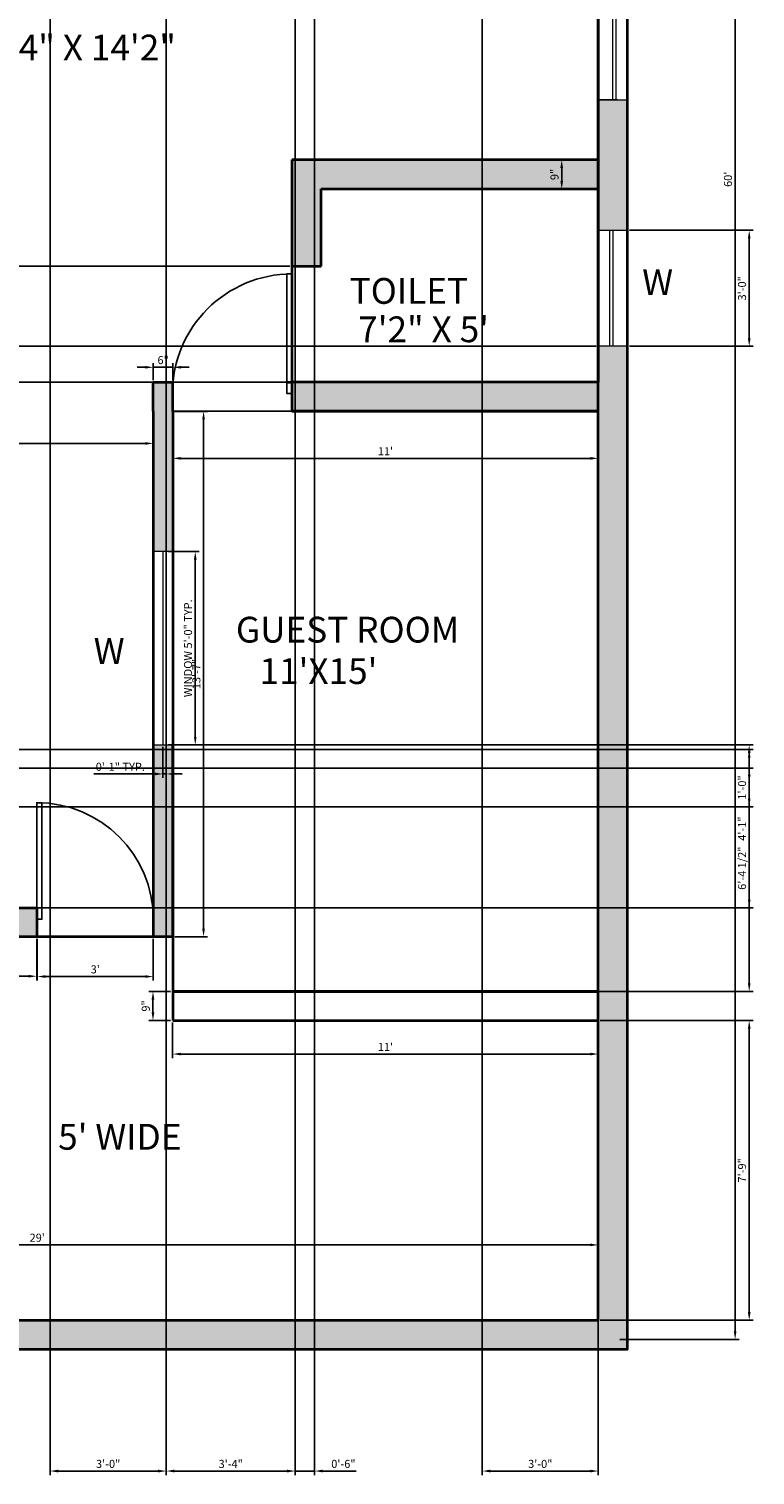
# Model space of a CAD drawing. Units: inches. Extents: x 844 to 1293, y 1224 to 2014.
# Tile 2 of 4: x 1068 to 1293, y 1224 to 1673. Entities that reach past the tile are written whole.
import ezdxf

# ---------------------------------------------------------------- set-up
doc = ezdxf.new("R2010")
doc.units = ezdxf.units.IN
for name, color, linetype, lineweight in [('A-ANNO-DIMS', 2, 'Continuous', 18), ('A-ANNO-TEXT', 3, 'Continuous', 18), ('A-AREA-IDEN', 7, 'Continuous', 25), ('A-DOOR', 3, 'Continuous', 25), ('A-GLAZ', 4, 'Continuous', 18), ('A-WALL', 7, 'Continuous', 35), ('A-WALL-PATT', 252, 'Continuous', 13)]:
    doc.layers.add(name, color=color, linetype=linetype, lineweight=lineweight)
doc.styles.get("Standard").update_dxf_attribs({"font": 'arial.ttf'})
doc.dimstyles.new('Copy of ISO-25', dxfattribs={"dimtxt": 2.5, "dimasz": 2.5, "dimexe": 1.25, "dimexo": 0.625, "dimtad": 1, "dimlunit": 4, "dimtxsty": 'Standard', "dimcen": 2.5, "dimadec": 0, "dimazin": 0, "dimtfac": 1, "dimtmove": 0, "dimatfit": 3, "dimfxl": 1, "dimarcsym": 0})

# ---------------------------------------------------------------- blocks, each defined once
blk = doc.blocks.new('*U3')
for p, q in [((0, 0), (0, -6)), ((40, 0), (40, -6))]:
    blk.add_line(p, q)
blk.add_lwpolyline([(0, 0), (0, 40), (1.75, 40), (1.75, 0)], close=True)
blk.add_arc((0, 0), 40, 0, 90)
blk = doc.blocks.new('*U2')
for p, q in [((0, 0), (0, -6)), ((-40, 0), (-40, -6))]:
    blk.add_line(p, q)
blk.add_lwpolyline([(0, 0), (0, 40), (-1.75, 40), (-1.75, 0)], close=True)
blk.add_arc((0, 0), 40, 90, 180)
blk = doc.blocks.new('*D17')
at = {"layer": 'A-ANNO-DIMS', "color": 0, "lineweight": -2, "transparency": 16777216}
for p, q in [((998.46, 1553.35), (998.46, 1542.83)), ((1106.46, 1553.35), (1106.46, 1542.83)), ((1000.96, 1544.08), (1103.96, 1544.08))]:
    blk.add_line(p, q, dxfattribs=at)
at = {"layer": 'A-ANNO-DIMS', "color": 0, "transparency": 16777216}
for points in [[(1000.96, 1544.49), (1000.96, 1543.66), (998.46, 1544.08)], [(1103.96, 1544.49), (1103.96, 1543.66), (1106.46, 1544.08)]]:
    blk.add_solid(points, dxfattribs=at)
at = {"layer": 'Defpoints', "color": 0, "transparency": 16777216}
for p in [(998.46, 1553.98), (1106.46, 1553.98), (1106.46, 1544.08)]:
    blk.add_point(p, dxfattribs=at)
at = {"layer": 'A-ANNO-DIMS', "color": 0, "transparency": 16777216, "insert": (1052.46, 1545.98), "char_height": 2.5, "attachment_point": 5}
blk.add_mtext("9'", dxfattribs=at)
blk = doc.blocks.new('*D20')
at = {"layer": 'A-ANNO-DIMS', "color": 0, "lineweight": -2, "transparency": 16777216}
for p, q in [((1251.09, 1986.04), (1288.15, 1986.04)), ((1286.9, 1983.54), (1286.9, 1268.54)), ((1251.09, 1266.04), (1288.15, 1266.04))]:
    blk.add_line(p, q, dxfattribs=at)
at = {"layer": 'A-ANNO-DIMS', "color": 0, "transparency": 16777216}
for points in [[(1286.48, 1983.54), (1287.31, 1983.54), (1286.9, 1986.04)], [(1286.48, 1268.54), (1287.31, 1268.54), (1286.9, 1266.04)]]:
    blk.add_solid(points, dxfattribs=at)
at = {"layer": 'Defpoints', "color": 0, "transparency": 16777216}
for p in [(1250.46, 1986.04), (1250.46, 1266.04), (1286.9, 1266.04)]:
    blk.add_point(p, dxfattribs=at)
at = {"layer": 'A-ANNO-DIMS', "color": 0, "transparency": 16777216, "insert": (1285, 1626.04), "char_height": 2.5, "attachment_point": 5, "rotation": 90}
blk.add_mtext("60'", dxfattribs=at)
blk = doc.blocks.new('*D21')
at = {"layer": 'A-ANNO-DIMS', "color": 0, "lineweight": -2, "transparency": 16777216}
for p, q in [((989.46, 1390.05), (989.46, 1377.52)), ((1070.31, 1390.42), (1070.31, 1377.52)), ((991.96, 1378.77), (1067.81, 1378.77))]:
    blk.add_line(p, q, dxfattribs=at)
at = {"layer": 'A-ANNO-DIMS', "color": 0, "transparency": 16777216}
for points in [[(991.96, 1379.19), (991.96, 1378.36), (989.46, 1378.77)], [(1067.81, 1379.19), (1067.81, 1378.36), (1070.31, 1378.77)]]:
    blk.add_solid(points, dxfattribs=at)
at = {"layer": 'Defpoints', "color": 0, "transparency": 16777216}
for p in [(1070.31, 1391.04), (989.46, 1390.68), (1070.31, 1378.77)]:
    blk.add_point(p, dxfattribs=at)
at = {"layer": 'A-ANNO-DIMS', "color": 0, "transparency": 16777216, "insert": (1029.89, 1382.36), "char_height": 2.5, "attachment_point": 5}
blk.add_mtext('6\'-8{\\H1x;\\S3/4;}"', dxfattribs=at)
blk = doc.blocks.new('*D22')
at = {"layer": 'A-ANNO-DIMS', "color": 0, "lineweight": -2, "transparency": 16777216}
for p, q in [((1070.46, 1390.42), (1070.46, 1377.42)), ((1106.46, 1390.42), (1106.46, 1377.42)), ((1072.96, 1378.67), (1103.96, 1378.67))]:
    blk.add_line(p, q, dxfattribs=at)
at = {"layer": 'A-ANNO-DIMS', "color": 0, "transparency": 16777216}
for points in [[(1072.96, 1379.09), (1072.96, 1378.26), (1070.46, 1378.67)], [(1103.96, 1379.09), (1103.96, 1378.26), (1106.46, 1378.67)]]:
    blk.add_solid(points, dxfattribs=at)
at = {"layer": 'Defpoints', "color": 0, "transparency": 16777216}
for p in [(1070.46, 1391.04), (1106.46, 1391.04), (1106.46, 1378.67)]:
    blk.add_point(p, dxfattribs=at)
at = {"layer": 'A-ANNO-DIMS', "color": 0, "transparency": 16777216, "insert": (1088.46, 1380.57), "char_height": 2.5, "attachment_point": 5}
blk.add_mtext("3'", dxfattribs=at)
blk = doc.blocks.new('*D23')
at = {"layer": 'A-ANNO-DIMS', "color": 0, "lineweight": -2, "transparency": 16777216}
for p, q in [((1111.84, 1374.04), (1105.1, 1374.04)), ((1106.35, 1367.54), (1106.35, 1371.54)), ((1111.84, 1365.04), (1105.1, 1365.04))]:
    blk.add_line(p, q, dxfattribs=at)
at = {"layer": 'A-ANNO-DIMS', "color": 0, "transparency": 16777216}
for points in [[(1105.93, 1371.54), (1106.77, 1371.54), (1106.35, 1374.04)], [(1105.93, 1367.54), (1106.77, 1367.54), (1106.35, 1365.04)]]:
    blk.add_solid(points, dxfattribs=at)
at = {"layer": 'Defpoints', "color": 0, "transparency": 16777216}
for p in [(1106.35, 1374.04), (1112.46, 1374.04), (1112.46, 1365.04)]:
    blk.add_point(p, dxfattribs=at)
at = {"layer": 'A-ANNO-DIMS', "color": 0, "transparency": 16777216, "insert": (1104.45, 1369.54), "char_height": 2.5, "attachment_point": 5, "rotation": 90}
blk.add_mtext('9"', dxfattribs=at)
blk = doc.blocks.new('*D24')
at = {"layer": 'A-ANNO-DIMS', "color": 0, "lineweight": -2, "transparency": 16777216}
for p, q in [((1112.46, 1364.42), (1112.46, 1353.37)), ((1244.46, 1364.42), (1244.46, 1353.37)), ((1114.96, 1354.62), (1241.96, 1354.62))]:
    blk.add_line(p, q, dxfattribs=at)
at = {"layer": 'A-ANNO-DIMS', "color": 0, "transparency": 16777216}
for points in [[(1114.96, 1355.04), (1114.96, 1354.2), (1112.46, 1354.62)], [(1241.96, 1355.04), (1241.96, 1354.2), (1244.46, 1354.62)]]:
    blk.add_solid(points, dxfattribs=at)
at = {"layer": 'Defpoints', "color": 0, "transparency": 16777216}
for p in [(1112.46, 1365.04), (1244.46, 1365.04), (1244.46, 1354.62)]:
    blk.add_point(p, dxfattribs=at)
at = {"layer": 'A-ANNO-DIMS', "color": 0, "transparency": 16777216, "insert": (1178.46, 1356.5), "char_height": 2.5, "attachment_point": 5}
blk.add_mtext("11'", dxfattribs=at)
blk = doc.blocks.new('*D31')
at = {"layer": 'A-ANNO-DIMS', "color": 0, "lineweight": -2, "transparency": 16777216}
for p, q in [((896.46, 1272.67), (896.46, 1296.66)), ((1241.96, 1295.41), (898.96, 1295.41)), ((1244.46, 1272.67), (1244.46, 1296.66))]:
    blk.add_line(p, q, dxfattribs=at)
at = {"layer": 'A-ANNO-DIMS', "color": 0, "transparency": 16777216}
for points in [[(898.96, 1295.83), (898.96, 1295), (896.46, 1295.41)], [(1241.96, 1295.83), (1241.96, 1295), (1244.46, 1295.41)]]:
    blk.add_solid(points, dxfattribs=at)
at = {"layer": 'Defpoints', "color": 0, "transparency": 16777216}
for p in [(896.46, 1295.41), (896.46, 1272.04), (1244.46, 1272.04)]:
    blk.add_point(p, dxfattribs=at)
at = {"layer": 'A-ANNO-DIMS', "color": 0, "transparency": 16777216, "insert": (1070.46, 1297.32), "char_height": 2.5, "attachment_point": 5}
blk.add_mtext("29'", dxfattribs=at)
blk = doc.blocks.new('*D32')
at = {"layer": 'A-ANNO-DIMS', "color": 0, "lineweight": -2, "transparency": 16777216}
for p, q in [((1112.46, 1553.42), (1112.46, 1538.2)), ((1244.46, 1553.42), (1244.46, 1538.2)), ((1114.96, 1539.45), (1241.96, 1539.45))]:
    blk.add_line(p, q, dxfattribs=at)
at = {"layer": 'A-ANNO-DIMS', "color": 0, "transparency": 16777216}
for points in [[(1114.96, 1539.87), (1114.96, 1539.04), (1112.46, 1539.45)], [(1241.96, 1539.87), (1241.96, 1539.04), (1244.46, 1539.45)]]:
    blk.add_solid(points, dxfattribs=at)
at = {"layer": 'Defpoints', "color": 0, "transparency": 16777216}
for p in [(1112.46, 1554.04), (1244.46, 1554.04), (1244.46, 1539.45)]:
    blk.add_point(p, dxfattribs=at)
at = {"layer": 'A-ANNO-DIMS', "color": 0, "transparency": 16777216, "insert": (1178.46, 1541.33), "char_height": 2.5, "attachment_point": 5}
blk.add_mtext("11'", dxfattribs=at)
blk = doc.blocks.new('*D33')
at = {"layer": 'A-ANNO-DIMS', "color": 0, "lineweight": -2, "transparency": 16777216}
for p, q in [((1113.09, 1554.04), (1123.29, 1554.04)), ((1122.04, 1551.54), (1122.04, 1393.54)), ((1113.09, 1391.04), (1123.29, 1391.04))]:
    blk.add_line(p, q, dxfattribs=at)
at = {"layer": 'A-ANNO-DIMS', "color": 0, "transparency": 16777216}
for points in [[(1121.62, 1551.54), (1122.46, 1551.54), (1122.04, 1554.04)], [(1121.62, 1393.54), (1122.46, 1393.54), (1122.04, 1391.04)]]:
    blk.add_solid(points, dxfattribs=at)
at = {"layer": 'Defpoints', "color": 0, "transparency": 16777216}
for p in [(1112.46, 1554.04), (1112.46, 1391.04), (1122.04, 1391.04)]:
    blk.add_point(p, dxfattribs=at)
at = {"layer": 'A-ANNO-DIMS', "color": 0, "transparency": 16777216, "insert": (1120.14, 1472.54), "char_height": 2.5, "attachment_point": 5, "rotation": 90}
blk.add_mtext('13\'-7"', dxfattribs=at)
blk = doc.blocks.new('*D38')
at = {"layer": 'A-ANNO-DIMS', "color": 0, "lineweight": -2, "transparency": 16777216}
for p, q in [((1103.96, 1567.71), (1101.46, 1567.71)), ((1106.46, 1563.67), (1106.46, 1568.96)), ((1112.55, 1567.71), (1106.46, 1567.71)), ((1112.55, 1563.67), (1112.55, 1568.96)), ((1115.05, 1567.71), (1117.55, 1567.71))]:
    blk.add_line(p, q, dxfattribs=at)
at = {"layer": 'A-ANNO-DIMS', "color": 0, "transparency": 16777216}
for points in [[(1103.96, 1568.13), (1103.96, 1567.29), (1106.46, 1567.71)], [(1115.05, 1568.13), (1115.05, 1567.29), (1112.55, 1567.71)]]:
    blk.add_solid(points, dxfattribs=at)
at = {"layer": 'Defpoints', "color": 0, "transparency": 16777216}
for p in [(1106.46, 1567.71), (1106.46, 1563.04), (1112.55, 1563.04)]:
    blk.add_point(p, dxfattribs=at)
at = {"layer": 'A-ANNO-DIMS', "color": 0, "transparency": 16777216, "insert": (1109.51, 1569.61), "char_height": 2.5, "attachment_point": 5}
blk.add_mtext('6"', dxfattribs=at)
blk = doc.blocks.new('*D41')
at = {"layer": 'A-ANNO-DIMS', "color": 0, "lineweight": -2, "transparency": 16777216}
for p, q in [((1243.84, 1632.04), (1231.86, 1632.04)), ((1233.11, 1625.54), (1233.11, 1629.54)), ((1243.84, 1623.04), (1231.86, 1623.04))]:
    blk.add_line(p, q, dxfattribs=at)
at = {"layer": 'A-ANNO-DIMS', "color": 0, "transparency": 16777216}
for points in [[(1232.69, 1629.54), (1233.53, 1629.54), (1233.11, 1632.04)], [(1232.69, 1625.54), (1233.53, 1625.54), (1233.11, 1623.04)]]:
    blk.add_solid(points, dxfattribs=at)
at = {"layer": 'Defpoints', "color": 0, "transparency": 16777216}
for p in [(1233.11, 1632.04), (1244.46, 1632.04), (1244.46, 1623.04)]:
    blk.add_point(p, dxfattribs=at)
at = {"layer": 'A-ANNO-DIMS', "color": 0, "transparency": 16777216, "insert": (1231.21, 1627.54), "char_height": 2.5, "attachment_point": 5, "rotation": 90}
blk.add_mtext('9"', dxfattribs=at)
blk = doc.blocks.new('WIN-GLAZ-60IN')
for p, q in [((0, 60), (0, 0)), ((1, 60), (1, 0))]:
    blk.add_line(p, q)
blk = doc.blocks.new('*D47')
at = {"layer": 'A-ANNO-DIMS', "color": 0, "lineweight": -2, "transparency": 16777216}
for p, q in [((1111.09, 1510.53), (1120.71, 1510.53)), ((1119.46, 1508.03), (1119.46, 1453.03)), ((1111.09, 1450.53), (1120.71, 1450.53))]:
    blk.add_line(p, q, dxfattribs=at)
at = {"layer": 'A-ANNO-DIMS', "color": 0, "transparency": 16777216}
for points in [[(1119.05, 1508.03), (1119.88, 1508.03), (1119.46, 1510.53)], [(1119.05, 1453.03), (1119.88, 1453.03), (1119.46, 1450.53)]]:
    blk.add_solid(points, dxfattribs=at)
at = {"layer": 'Defpoints', "color": 0, "transparency": 16777216}
for p in [(1110.46, 1510.53), (1110.46, 1450.53), (1119.46, 1450.53)]:
    blk.add_point(p, dxfattribs=at)
at = {"layer": 'A-ANNO-DIMS', "color": 0, "transparency": 16777216, "insert": (1117.55, 1480.53), "char_height": 2.5, "attachment_point": 5, "rotation": 90}
blk.add_mtext('WINDOW 5\'-0" TYP.', dxfattribs=at)
blk = doc.blocks.new('*D48')
at = {"layer": 'A-ANNO-DIMS', "color": 0, "lineweight": -2, "transparency": 16777216}
for p, q in [((1109.46, 1449.91), (1109.46, 1440.28)), ((1110.46, 1449.91), (1110.46, 1440.28)), ((1106.96, 1441.53), (1087.98, 1441.53)), ((1110.46, 1441.53), (1109.46, 1441.53)), ((1112.96, 1441.53), (1115.46, 1441.53))]:
    blk.add_line(p, q, dxfattribs=at)
at = {"layer": 'A-ANNO-DIMS', "color": 0, "transparency": 16777216}
for points in [[(1106.96, 1441.95), (1106.96, 1441.11), (1109.46, 1441.53)], [(1112.96, 1441.95), (1112.96, 1441.11), (1110.46, 1441.53)]]:
    blk.add_solid(points, dxfattribs=at)
at = {"layer": 'Defpoints', "color": 0, "transparency": 16777216}
for p in [(1109.46, 1450.53), (1110.46, 1450.53), (1109.46, 1441.53)]:
    blk.add_point(p, dxfattribs=at)
at = {"layer": 'A-ANNO-DIMS', "color": 0, "transparency": 16777216, "insert": (1096.22, 1443.43), "char_height": 2.5, "attachment_point": 5}
blk.add_mtext('0\'-1" TYP.', dxfattribs=at)
blk = doc.blocks.new('*D53')
at = {"layer": 'A-ANNO-DIMS', "color": 0, "lineweight": -2, "transparency": 16777216}
for p, q in [((1245.09, 1365.04), (1292.51, 1365.04)), ((1291.26, 1274.54), (1291.26, 1362.54)), ((1245.09, 1272.04), (1292.51, 1272.04))]:
    blk.add_line(p, q, dxfattribs=at)
at = {"layer": 'A-ANNO-DIMS', "color": 0, "transparency": 16777216}
for points in [[(1290.85, 1362.54), (1291.68, 1362.54), (1291.26, 1365.04)], [(1290.85, 1274.54), (1291.68, 1274.54), (1291.26, 1272.04)]]:
    blk.add_solid(points, dxfattribs=at)
at = {"layer": 'Defpoints', "color": 0, "transparency": 16777216}
for p in [(1244.46, 1365.04), (1291.26, 1365.04), (1244.46, 1272.04)]:
    blk.add_point(p, dxfattribs=at)
at = {"layer": 'A-ANNO-DIMS', "color": 0, "transparency": 16777216, "insert": (1289.36, 1318.54), "char_height": 2.5, "attachment_point": 5, "rotation": 90}
blk.add_mtext('7\'-9"', dxfattribs=at)
blk = doc.blocks.new('*D59')
at = {"layer": 'A-ANNO-DIMS', "color": 0, "lineweight": -2, "transparency": 16777216}
for p, q in [((1254.09, 1610.21), (1292.51, 1610.21)), ((1291.26, 1576.71), (1291.26, 1607.71)), ((1254.09, 1574.21), (1292.51, 1574.21))]:
    blk.add_line(p, q, dxfattribs=at)
at = {"layer": 'A-ANNO-DIMS', "color": 0, "transparency": 16777216}
for points in [[(1290.85, 1607.71), (1291.68, 1607.71), (1291.26, 1610.21)], [(1290.85, 1576.71), (1291.68, 1576.71), (1291.26, 1574.21)]]:
    blk.add_solid(points, dxfattribs=at)
at = {"layer": 'Defpoints', "color": 0, "transparency": 16777216}
for p in [(1253.46, 1610.21), (1291.26, 1610.21), (1253.46, 1574.21)]:
    blk.add_point(p, dxfattribs=at)
at = {"layer": 'A-ANNO-DIMS', "color": 0, "transparency": 16777216, "insert": (1289.36, 1592.21), "char_height": 2.5, "attachment_point": 5, "rotation": 90}
blk.add_mtext('3\'-0"', dxfattribs=at)
blk = doc.blocks.new('*D60')
at = {"layer": 'A-ANNO-DIMS', "color": 0, "lineweight": -2, "transparency": 16777216}
for p, q in [((1243.84, 1574.21), (848.41, 1574.21)), ((849.66, 1571.71), (849.66, 1565.54)), ((1243.84, 1563.04), (848.41, 1563.04))]:
    blk.add_line(p, q, dxfattribs=at)
at = {"layer": 'A-ANNO-DIMS', "color": 0, "transparency": 16777216}
for points in [[(849.25, 1571.71), (850.08, 1571.71), (849.66, 1574.21)], [(849.25, 1565.54), (850.08, 1565.54), (849.66, 1563.04)]]:
    blk.add_solid(points, dxfattribs=at)
at = {"layer": 'Defpoints', "color": 0, "transparency": 16777216}
for p in [(1244.46, 1574.21), (849.66, 1563.04), (1244.46, 1563.04)]:
    blk.add_point(p, dxfattribs=at)
at = {"layer": 'A-ANNO-DIMS', "color": 0, "transparency": 16777216, "insert": (847.76, 1568.63), "char_height": 2.5, "attachment_point": 5, "rotation": 90}
blk.add_mtext('0\'-11"', dxfattribs=at)
blk = doc.blocks.new('*D61')
at = {"layer": 'A-ANNO-DIMS', "color": 0, "lineweight": -2, "transparency": 16777216}
for p, q in [((999.09, 1449.1), (1292.51, 1449.1)), ((1291.26, 1402.54), (1291.26, 1446.6)), ((999.09, 1400.04), (1292.51, 1400.04))]:
    blk.add_line(p, q, dxfattribs=at)
at = {"layer": 'A-ANNO-DIMS', "color": 0, "transparency": 16777216}
for points in [[(1290.85, 1446.6), (1291.68, 1446.6), (1291.26, 1449.1)], [(1290.85, 1402.54), (1291.68, 1402.54), (1291.26, 1400.04)]]:
    blk.add_solid(points, dxfattribs=at)
at = {"layer": 'Defpoints', "color": 0, "transparency": 16777216}
for p in [(998.46, 1449.1), (1291.26, 1449.1), (998.46, 1400.04)]:
    blk.add_point(p, dxfattribs=at)
at = {"layer": 'A-ANNO-DIMS', "color": 0, "transparency": 16777216, "insert": (1289.38, 1424.57), "char_height": 2.5, "attachment_point": 5, "rotation": 90}
blk.add_mtext('4\'-1"', dxfattribs=at)
blk = doc.blocks.new('*D62')
at = {"layer": 'A-ANNO-DIMS', "color": 0, "lineweight": -2, "transparency": 16777216}
for p, q in [((1113.09, 1450.53), (1292.51, 1450.53)), ((1291.26, 1376.54), (1291.26, 1448.03)), ((1113.09, 1374.04), (1292.51, 1374.04))]:
    blk.add_line(p, q, dxfattribs=at)
at = {"layer": 'A-ANNO-DIMS', "color": 0, "transparency": 16777216}
for points in [[(1290.85, 1448.03), (1291.68, 1448.03), (1291.26, 1450.53)], [(1290.85, 1376.54), (1291.68, 1376.54), (1291.26, 1374.04)]]:
    blk.add_solid(points, dxfattribs=at)
at = {"layer": 'Defpoints', "color": 0, "transparency": 16777216}
for p in [(1112.46, 1450.53), (1291.26, 1450.53), (1112.46, 1374.04)]:
    blk.add_point(p, dxfattribs=at)
at = {"layer": 'A-ANNO-DIMS', "color": 0, "transparency": 16777216, "insert": (1289.35, 1412.29), "char_height": 2.5, "attachment_point": 5, "rotation": 90}
blk.add_mtext('6\'-4 1/2"', dxfattribs=at)
blk = doc.blocks.new('*D63')
at = {"layer": 'A-ANNO-DIMS', "color": 0, "lineweight": -2, "transparency": 16777216}
for p, q in [((1110.46, 1910.42), (1110.46, 1223.99)), ((1150.46, 1910.42), (1150.46, 1223.99)), ((1112.96, 1225.24), (1147.96, 1225.24))]:
    blk.add_line(p, q, dxfattribs=at)
at = {"layer": 'A-ANNO-DIMS', "color": 0, "transparency": 16777216}
for points in [[(1112.96, 1225.66), (1112.96, 1224.82), (1110.46, 1225.24)], [(1147.96, 1225.66), (1147.96, 1224.82), (1150.46, 1225.24)]]:
    blk.add_solid(points, dxfattribs=at)
at = {"layer": 'Defpoints', "color": 0, "transparency": 16777216}
for p in [(1110.46, 1911.04), (1150.46, 1911.04), (1150.46, 1225.24)]:
    blk.add_point(p, dxfattribs=at)
at = {"layer": 'A-ANNO-DIMS', "color": 0, "transparency": 16777216, "insert": (1130.46, 1227.14), "char_height": 2.5, "attachment_point": 5}
blk.add_mtext('3\'-4"', dxfattribs=at)
blk = doc.blocks.new('*D64')
at = {"layer": 'A-ANNO-DIMS', "color": 0, "lineweight": -2, "transparency": 16777216}
for p, q in [((1208.46, 1910.42), (1208.46, 1223.99)), ((1244.46, 1910.42), (1244.46, 1223.99)), ((1210.96, 1225.24), (1241.96, 1225.24))]:
    blk.add_line(p, q, dxfattribs=at)
at = {"layer": 'A-ANNO-DIMS', "color": 0, "transparency": 16777216}
for points in [[(1210.96, 1225.66), (1210.96, 1224.82), (1208.46, 1225.24)], [(1241.96, 1225.66), (1241.96, 1224.82), (1244.46, 1225.24)]]:
    blk.add_solid(points, dxfattribs=at)
at = {"layer": 'Defpoints', "color": 0, "transparency": 16777216}
for p in [(1208.46, 1911.04), (1244.46, 1911.04), (1244.46, 1225.24)]:
    blk.add_point(p, dxfattribs=at)
at = {"layer": 'A-ANNO-DIMS', "color": 0, "transparency": 16777216, "insert": (1226.46, 1227.14), "char_height": 2.5, "attachment_point": 5}
blk.add_mtext('3\'-0"', dxfattribs=at)
blk = doc.blocks.new('*D67')
at = {"layer": 'A-ANNO-DIMS', "color": 0, "lineweight": -2, "transparency": 16777216}
for p, q in [((1074.46, 1732.42), (1074.46, 1223.99)), ((1110.46, 1732.42), (1110.46, 1223.99)), ((1076.96, 1225.24), (1107.96, 1225.24))]:
    blk.add_line(p, q, dxfattribs=at)
at = {"layer": 'A-ANNO-DIMS', "color": 0, "transparency": 16777216}
for points in [[(1076.96, 1225.66), (1076.96, 1224.82), (1074.46, 1225.24)], [(1107.96, 1225.66), (1107.96, 1224.82), (1110.46, 1225.24)]]:
    blk.add_solid(points, dxfattribs=at)
at = {"layer": 'Defpoints', "color": 0, "transparency": 16777216}
for p in [(1074.46, 1733.04), (1110.46, 1733.04), (1110.46, 1225.24)]:
    blk.add_point(p, dxfattribs=at)
at = {"layer": 'A-ANNO-DIMS', "color": 0, "transparency": 16777216, "insert": (1092.46, 1227.14), "char_height": 2.5, "attachment_point": 5}
blk.add_mtext('3\'-0"', dxfattribs=at)
blk = doc.blocks.new('*D68')
at = {"layer": 'A-ANNO-DIMS', "color": 0, "lineweight": -2, "transparency": 16777216}
for p, q in [((1148.84, 1599.04), (848.41, 1599.04)), ((849.66, 1565.54), (849.66, 1596.54)), ((1148.84, 1563.04), (848.41, 1563.04))]:
    blk.add_line(p, q, dxfattribs=at)
at = {"layer": 'A-ANNO-DIMS', "color": 0, "transparency": 16777216}
for points in [[(849.25, 1596.54), (850.08, 1596.54), (849.66, 1599.04)], [(849.25, 1565.54), (850.08, 1565.54), (849.66, 1563.04)]]:
    blk.add_solid(points, dxfattribs=at)
at = {"layer": 'Defpoints', "color": 0, "transparency": 16777216}
for p in [(849.66, 1599.04), (1149.46, 1599.04), (1149.46, 1563.04)]:
    blk.add_point(p, dxfattribs=at)
at = {"layer": 'A-ANNO-DIMS', "color": 0, "transparency": 16777216, "insert": (847.76, 1581.04), "char_height": 2.5, "attachment_point": 5, "rotation": 90}
blk.add_mtext('3\'-0"', dxfattribs=at)
blk = doc.blocks.new('*D71')
at = {"layer": 'A-ANNO-DIMS', "color": 0, "lineweight": -2, "transparency": 16777216}
for p, q in [((933.09, 1443.33), (1292.51, 1443.33)), ((1291.26, 1433.83), (1291.26, 1440.83)), ((933.09, 1431.33), (1292.51, 1431.33))]:
    blk.add_line(p, q, dxfattribs=at)
at = {"layer": 'A-ANNO-DIMS', "color": 0, "transparency": 16777216}
for points in [[(1290.85, 1440.83), (1291.68, 1440.83), (1291.26, 1443.33)], [(1290.85, 1433.83), (1291.68, 1433.83), (1291.26, 1431.33)]]:
    blk.add_solid(points, dxfattribs=at)
at = {"layer": 'Defpoints', "color": 0, "transparency": 16777216}
for p in [(932.46, 1443.33), (1291.26, 1443.33), (932.46, 1431.33)]:
    blk.add_point(p, dxfattribs=at)
at = {"layer": 'A-ANNO-DIMS', "color": 0, "transparency": 16777216, "insert": (1289.36, 1437.33), "char_height": 2.5, "attachment_point": 5, "rotation": 90}
blk.add_mtext('1\'-0"', dxfattribs=at)
blk = doc.blocks.new('*D73')
at = {"layer": 'A-ANNO-DIMS', "color": 0, "lineweight": -2, "transparency": 16777216}
for p, q in [((1150.46, 1919.42), (1150.46, 1223.99)), ((1156.46, 1919.42), (1156.46, 1223.99)), ((1147.96, 1225.24), (1145.46, 1225.24)), ((1150.46, 1225.24), (1156.46, 1225.24)), ((1158.96, 1225.24), (1169.36, 1225.24))]:
    blk.add_line(p, q, dxfattribs=at)
at = {"layer": 'A-ANNO-DIMS', "color": 0, "transparency": 16777216}
for points in [[(1147.96, 1225.66), (1147.96, 1224.82), (1150.46, 1225.24)], [(1158.96, 1225.66), (1158.96, 1224.82), (1156.46, 1225.24)]]:
    blk.add_solid(points, dxfattribs=at)
at = {"layer": 'Defpoints', "color": 0, "transparency": 16777216}
for p in [(1150.46, 1920.04), (1156.46, 1920.04), (1156.46, 1225.24)]:
    blk.add_point(p, dxfattribs=at)
at = {"layer": 'A-ANNO-DIMS', "color": 0, "transparency": 16777216, "insert": (1165.41, 1227.14), "char_height": 2.5, "attachment_point": 5}
blk.add_mtext('0\'-6"', dxfattribs=at)

msp = doc.modelspace()

# ---------------------------------------------------------------- hatches: boundary and pattern name
at = {"layer": 'A-WALL-PATT'}
h = msp.add_hatch(color=256, dxfattribs=at)
h.dxf.hatch_style = 1
h.paths.add_polyline_path([(1253.465, 1989.042), (887.465, 1989.042), (887.465, 1920.042), (887.465, 1911.042), (887.465, 1871.621), (896.465, 1871.621), (896.465, 1911.042), (896.465, 1920.042), (896.465, 1980.042), (1000.465, 1980.042), (1244.465, 1980.042), (1244.465, 1968.042), (1253.465, 1968.042)])
h.paths.add_polyline_path([(1006.465, 1944.042), (1000.465, 1944.042), (1000.465, 1920.042), (896.465, 1920.042), (896.465, 1911.042), (1006.465, 1911.042), (1006.465, 1920.042)], flags=17)
h.paths.add_polyline_path([(1253.465, 1968.042), (1244.465, 1968.042), (1244.465, 1932.042), (1253.465, 1932.042)], flags=17)
h.paths.add_polyline_path([(1253.465, 1920.042), (1253.465, 1932.042), (1244.465, 1932.042), (1244.465, 1920.042), (1244.465, 1911.042), (1244.465, 1884.775), (1253.465, 1884.775), (1253.465, 1911.042)], flags=17)
h.paths.add_polyline_path([(1208.465, 1920.042), (1156.465, 1920.042), (1156.465, 1980.042), (1150.465, 1980.042), (1150.465, 1920.042), (1150.465, 1911.042), (1208.465, 1911.042)], flags=17)
h.paths.add_polyline_path([(1110.465, 1920.042), (1074.465, 1920.042), (1074.465, 1911.042), (1110.465, 1911.042)], flags=17)
h.paths.add_polyline_path([(896.465, 1811.621), (887.465, 1811.621), (887.465, 1672.343), (896.465, 1672.343), (896.465, 1733.042), (896.465, 1742.042)])
h.paths.add_polyline_path([(896.465, 1624.343), (887.465, 1624.343), (887.465, 1263.042), (1253.465, 1263.042), (1253.465, 1574.212), (1244.465, 1574.212), (1244.465, 1563.042), (1244.465, 1554.042), (1244.465, 1272.042), (1016.465, 1272.042), (1016.465, 1267.542), (896.465, 1267.542), (896.465, 1272.042), (896.465, 1554.042), (968.465, 1554.042), (989.465, 1554.042), (998.465, 1554.042), (998.465, 1623.042), (989.465, 1623.042), (989.465, 1563.042), (896.465, 1563.042)])
h.paths.add_polyline_path([(998.465, 1518.042), (994.855, 1518.042), (989.465, 1518.042), (989.465, 1497.104), (998.465, 1497.104)], flags=17)
h.paths.add_polyline_path([(998.465, 1449.104), (989.465, 1449.104), (989.465, 1391.042), (998.465, 1391.042), (1070.313, 1391.042), (1070.313, 1396.464), (1070.313, 1400.042), (998.465, 1400.042)], flags=17)
h.paths.add_polyline_path([(1112.465, 1450.531), (1106.465, 1450.531), (1106.465, 1400.042), (1106.465, 1391.042), (1112.465, 1391.042)], flags=17)
h.paths.add_polyline_path([(1112.465, 1554.042), (1112.394, 1554.042), (1112.394, 1559.602, -0.015479), (1112.465, 1561.896), (1112.465, 1563.042), (1106.465, 1563.042), (1106.465, 1554.042), (1106.465, 1510.531), (1112.465, 1510.531)], flags=17)
h.paths.add_polyline_path([(1158.465, 1623.042), (1244.465, 1623.042), (1244.465, 1632.042), (1158.465, 1632.042), (1149.465, 1632.042), (1149.465, 1599.042), (1158.465, 1599.042)])
h.paths.add_polyline_path([(1244.465, 1563.042), (1158.465, 1563.042), (1149.465, 1563.042), (1149.465, 1554.042), (1244.465, 1554.042)], flags=17)
h.paths.add_polyline_path([(1253.465, 1650.728), (1244.465, 1650.728), (1244.465, 1610.212), (1253.465, 1610.212)])
h.paths.add_polyline_path([(998.465, 1733.042), (989.465, 1733.042), (989.465, 1673.042), (998.465, 1673.042)])
h.paths.add_polyline_path([(1029.465, 1742.042), (896.465, 1742.042), (896.465, 1733.042), (989.465, 1733.042), (1029.465, 1733.042)])
h.paths.add_polyline_path([(1244.465, 1742.042), (1110.465, 1742.042), (1110.465, 1739.692, -0.0113533), (1110.5, 1738.147), (1110.5, 1733.042), (1244.465, 1733.042)])
h.paths.add_polyline_path([(1253.465, 1812.775), (1244.465, 1812.775), (1244.465, 1710.728), (1253.465, 1710.728)])
h.paths.add_polyline_path([(1074.465, 1911.042), (1074.465, 1920.042), (1065.465, 1920.042), (1065.465, 1911.042), (1065.465, 1742.042), (1065.465, 1733.042), (1074.465, 1733.042), (1074.465, 1742.042)])
h.paths.add_polyline_path([(1067.758, 1736.261), (1072.19, 1736.261), (1072.19, 1741.413), (1067.758, 1741.413)], flags=24)
h.paths.add_polyline_path([(975.783, 1886.472), (985.93, 1886.472), (985.93, 1891.624), (975.783, 1891.624)], flags=25)
h.paths.add_polyline_path([(917.205, 1821.36), (917.205, 1831.507), (912.053, 1831.507), (912.053, 1821.36)], flags=9)
h.paths.add_polyline_path([(1050.545, 1543.381), (1054.404, 1543.381), (1054.404, 1548.533), (1050.545, 1548.533)], flags=25)
h.paths.add_polyline_path([(1116.422, 1711.778), (1126.569, 1711.778), (1126.569, 1716.93), (1116.422, 1716.93)], flags=9)
h.paths.add_polyline_path([(1019.298, 1637.389), (1019.298, 1649.478), (1014.146, 1649.478), (1014.146, 1637.389)], flags=9)
h.paths.add_polyline_path([(980.864, 1534.121), (980.864, 1537.98), (975.712, 1537.98), (975.712, 1534.121)], flags=25)
h.paths.add_polyline_path([(1019.234, 1470.889), (1019.234, 1482.978), (1014.082, 1482.978), (1014.082, 1470.889)], flags=25)
h.paths.add_polyline_path([(1175.456, 1538.714), (1181.257, 1538.714), (1181.257, 1543.865), (1175.456, 1543.865)], flags=25)
h.paths.add_polyline_path([(1122.736, 1467.36), (1122.736, 1477.507), (1117.584, 1477.507), (1117.584, 1467.36)], flags=25)
h.paths.add_polyline_path([(907.276, 1556.335), (907.276, 1560.767), (902.124, 1560.767), (902.124, 1556.335)], flags=24)
h.paths.add_polyline_path([(1107.309, 1567.013), (1111.742, 1567.013), (1111.742, 1572.165), (1107.309, 1572.165)], flags=25)
h.paths.add_polyline_path([(955.783, 1784.038), (965.93, 1784.038), (965.93, 1789.19), (955.783, 1789.19)], flags=9)
h.paths.add_polyline_path([(1004.344, 1643.999), (1004.344, 1652.203), (999.192, 1652.203), (999.192, 1643.999)], flags=9)
h.paths.add_polyline_path([(973.263, 1534.121), (973.263, 1537.98), (968.111, 1537.98), (968.111, 1534.121)], flags=25)
h.paths.add_polyline_path([(1047.536, 1660.728), (1114.78, 1660.728), (1114.78, 1672.982), (1047.536, 1672.982)], flags=9)
h.paths.add_polyline_path([(1047.509, 1673.552), (1128.636, 1673.552), (1128.636, 1685.969), (1047.509, 1685.969)], flags=9)
h.paths.add_polyline_path([(999.825, 1474.75), (1014.374, 1474.75), (1014.374, 1486.75), (999.825, 1486.75)], flags=25)
h.paths.add_polyline_path([(1085.974, 1473.689), (1100.523, 1473.689), (1100.523, 1485.689), (1085.974, 1485.689)], flags=25)
h.paths.add_polyline_path([(898.914, 1844.786), (913.462, 1844.786), (913.462, 1856.786), (898.914, 1856.786)], flags=9)
h.paths.add_polyline_path([(1021.801, 1899.15), (1036.35, 1899.15), (1036.35, 1911.15), (1021.801, 1911.15)], flags=25)
h.paths.add_polyline_path([(933.371, 1817.465), (997.445, 1817.465), (997.445, 1829.522), (933.371, 1829.522)], flags=9)
h.paths.add_polyline_path([(912.536, 1375.627), (960.277, 1375.627), (960.277, 1387.881), (912.536, 1387.881)], flags=25)
h.paths.add_polyline_path([(908.723, 1393.944), (979.923, 1393.944), (979.923, 1406.361), (908.723, 1406.361)], flags=25)
h.paths.add_polyline_path([(907.199, 1415.111), (926.792, 1415.111), (926.792, 1427.316), (907.199, 1427.316)], flags=25)
h.paths.add_polyline_path([(1130.034, 1467.266), (1180.017, 1467.266), (1180.017, 1479.52), (1130.034, 1479.52)], flags=25)
h.paths.add_polyline_path([(1130.007, 1480.09), (1210.517, 1480.09), (1210.517, 1492.508), (1130.007, 1492.508)], flags=25)
h.paths.add_polyline_path([(918.552, 1280.947), (1012.38, 1280.947), (1012.38, 1293.356), (918.552, 1293.356)], flags=25)
h.paths.add_polyline_path([(1074.912, 1322.783), (1119.613, 1322.783), (1119.613, 1334.988), (1074.912, 1334.988)], flags=25)
h.paths.add_polyline_path([(994.568, 1321.709), (1075.078, 1321.709), (1075.078, 1334.127), (994.568, 1334.127)], flags=25)
h.paths.add_polyline_path([(932.502, 1835.432), (1188.778, 1835.432), (1188.778, 1847.849), (932.502, 1847.849)], flags=9)

# ---------------------------------------------------------------- linework, layer by layer
at = {"layer": 'A-DOOR'}
msp.add_line((1149.465, 1554.042), (1112.394, 1554.042), dxfattribs=at)
at = {"layer": 'A-GLAZ'}
for p, q in [((1250.465, 1650.728), (1244.465, 1650.728)), ((1244.465, 1650.728), (1253.465, 1650.728)), ((1244.465, 1610.212), (1253.465, 1610.212)), ((1247.965, 1610.212), (1247.965, 1574.212)), ((1248.965, 1610.212), (1248.965, 1574.212)), ((1253.465, 1610.212), (1253.465, 1574.212)), ((1253.465, 1574.212), (1244.465, 1574.212)), ((1112.465, 1510.531), (1106.465, 1510.531)), ((1106.465, 1510.531), (1106.465, 1450.531)), ((1112.465, 1450.531), (1112.465, 1510.531)), ((1106.465, 1450.531), (1112.465, 1450.531))]:
    msp.add_line(p, q, dxfattribs=at)
at = {"layer": 'A-WALL'}
for p, q in [((1244.465, 1733.042), (1244.465, 1563.042)), ((1158.465, 1632.042), (1149.465, 1632.042)), ((1149.465, 1632.042), (1149.465, 1563.042)), ((1244.465, 1632.042), (1158.465, 1632.042)), ((1244.465, 1623.042), (1244.465, 1632.042)), ((1158.465, 1599.042), (1158.465, 1623.042)), ((1158.465, 1623.042), (1244.465, 1623.042)), ((1244.465, 1623.042), (1244.465, 1610.212)), ((1149.465, 1599.042), (1158.465, 1599.042)), ((1106.465, 1554.042), (1106.465, 1563.042)), ((1106.465, 1563.042), (1112.554, 1563.042)), ((1112.465, 1554.042), (1112.465, 1563.042)), ((1112.465, 1563.042), (1112.465, 1563.042)), ((1147.843, 1563.042), (1149.465, 1563.042)), ((1149.465, 1563.042), (1149.465, 1554.042)), ((1158.465, 1563.042), (1149.465, 1563.042)), ((1244.465, 1563.042), (1158.465, 1563.042)), ((1244.465, 1563.042), (1158.465, 1563.042)), ((1244.465, 1554.042), (1244.465, 1563.042)), ((1106.465, 1554.042), (1106.465, 1400.042)), ((1112.465, 1554.042), (1112.465, 1400.042)), ((1112.465, 1554.042), (1112.465, 1374.042)), ((1149.465, 1554.042), (1244.465, 1554.042)), ((1244.465, 1554.042), (1149.465, 1554.042)), ((1112.465, 1391.042), (1112.465, 1450.531)), ((998.465, 1400.042), (1070.465, 1400.042)), ((1070.465, 1391.042), (1070.465, 1400.042)), ((1106.465, 1400.042), (1106.465, 1391.042)), ((1112.465, 1400.042), (1112.465, 1391.042)), ((1112.465, 1391.042), (998.465, 1391.042)), ((1106.465, 1391.042), (1070.465, 1391.042)), ((1112.465, 1374.042), (1244.465, 1374.042)), ((1112.465, 1374.042), (1112.465, 1365.042)), ((1244.465, 1374.042), (1112.465, 1374.042)), ((1112.465, 1374.042), (1112.465, 1365.042)), ((1244.465, 1365.042), (1244.465, 1374.042)), ((1112.465, 1365.042), (1244.465, 1365.042)), ((1112.465, 1365.042), (1244.465, 1365.042))]:
    msp.add_line(p, q, dxfattribs=at)
for points in [[(887.465, 1911.042), (887.465, 1263.042), (1253.465, 1263.042), (1253.465, 1911.042)], [(1016.465, 1272.042), (1244.465, 1272.042), (1244.465, 1911.042)]]:
    msp.add_lwpolyline(points, dxfattribs=at)

# ---------------------------------------------------------------- block references
at = {"layer": 'A-DOOR'}
for name, p, xscale, yscale, zscale in [('*U2', (1149.465, 1559.602), 0.9267755929778981, 0.9267755929778981, 0.9267755929778981), ('*U3', (1070.313, 1396.464), 0.9037906379330733, 0.9037906379330733, 0.9037906379330733)]:
    msp.add_blockref(name, p, dxfattribs=dict(at, xscale=xscale, yscale=yscale, zscale=zscale))
at = {"layer": 'A-GLAZ', "rotation": 180}
for p in [(1249.965, 1710.728), (1110.465, 1510.531)]:
    msp.add_blockref('WIN-GLAZ-60IN', p, dxfattribs=at)

# ---------------------------------------------------------------- texts
at = {"layer": 'A-ANNO-TEXT'}
for p in [(1258.065, 1590.125), (1087.974, 1475.689)]:
    msp.add_text('W', height=8, dxfattribs=at).set_placement(p)
at = {"layer": 'A-AREA-IDEN'}
for s, p in [('20\'4" X 14\'2"', (1049.578, 1662.907)), ('TOILET', (1167.355, 1587.399)), ('7\'2" X 5\'', (1169.998, 1575.488)), ('GUEST ROOM', (1132.076, 1482.296)), ("   11'X15'", (1132.076, 1469.445)), ("5' WIDE", (1076.946, 1324.954))]:
    msp.add_text(s, height=8, dxfattribs=at).set_placement(p)

# ---------------------------------------------------------------- dimensions: what is measured, and where the dimension line sits
at = {"layer": 'A-ANNO-DIMS'}
for base, p1, p2, override, picture, middle in [((1286.898, 1266.042), (1250.465, 1986.042), (1250.465, 1266.042), {"dimclrd": 0, "dimclre": 0, "dimclrt": 0}, '*D20', (1284.997, 1626.042)), ((1233.111, 1632.042), (1244.465, 1623.042), (1244.465, 1632.042), {"dimclrd": 0, "dimclre": 0, "dimclrt": 0}, '*D41', (1231.21, 1627.542)), ((1291.265, 1610.212), (1253.465, 1574.212), (1253.465, 1610.212), {"dimdec": 1, "dimlfac": 1, "dimrnd": 0, "dimzin": 1, "dimdsep": 46, "dimlunit": 4, "dimfrac": 2}, '*D59', (1289.363, 1592.212)), ((849.665, 1599.042), (1149.465, 1563.042), (1149.465, 1599.042), {"dimdec": 1, "dimlfac": 1, "dimrnd": 0, "dimzin": 1, "dimdsep": 46, "dimlunit": 4, "dimfrac": 2}, '*D68', (847.763, 1581.042)), ((849.665, 1563.042), (1244.465, 1574.212), (1244.465, 1563.042), {"dimdec": 1, "dimlfac": 1, "dimrnd": 0, "dimzin": 1, "dimdsep": 46, "dimlunit": 4, "dimfrac": 2}, '*D60', (847.763, 1568.627)), ((1122.04, 1391.042), (1112.465, 1554.042), (1112.465, 1391.042), {"dimclrd": 0, "dimclre": 0, "dimclrt": 0}, '*D33', (1120.138, 1472.542)), ((1291.265, 1450.531), (1112.465, 1374.042), (1112.465, 1450.531), {"dimdec": 1, "dimlfac": 1, "dimrnd": 0, "dimzin": 1, "dimdsep": 46, "dimlunit": 4, "dimfrac": 2}, '*D62', (1289.347, 1412.286)), ((1291.265, 1449.104), (998.465, 1400.042), (998.465, 1449.104), {"dimdec": 1, "dimlfac": 1, "dimrnd": 0, "dimzin": 1, "dimdsep": 46, "dimlunit": 4, "dimfrac": 2}, '*D61', (1289.385, 1424.573)), ((1291.265, 1443.328), (932.465, 1431.328), (932.465, 1443.328), {"dimdec": 1, "dimlfac": 1, "dimrnd": 0, "dimzin": 1, "dimdsep": 46, "dimlunit": 4, "dimfrac": 2}, '*D71', (1289.363, 1437.328)), ((1106.349, 1374.042), (1112.465, 1365.042), (1112.465, 1374.042), {"dimclrd": 0, "dimclre": 0, "dimclrt": 0}, '*D23', (1104.447, 1369.542)), ((1291.265, 1365.042), (1244.465, 1272.042), (1244.465, 1365.042), {"dimdec": 1, "dimlfac": 1, "dimrnd": 0, "dimzin": 1, "dimdsep": 46, "dimlunit": 4, "dimfrac": 2}, '*D53', (1289.363, 1318.542))]:
    dim = msp.add_linear_dim(base=base, p1=p1, p2=p2, angle=90, dimstyle='Copy of ISO-25', override=override, dxfattribs=at)
    dim.commit()
    dim.dimension.update_dxf_attribs({"geometry": picture, "text_midpoint": middle})
for base, p1, p2, override, picture, middle in [((1156.465, 1225.242), (1150.465, 1920.042), (1156.465, 1920.042), {"dimdec": 1, "dimlfac": 1, "dimrnd": 0, "dimzin": 1, "dimdsep": 46, "dimlunit": 4, "dimfrac": 2}, '*D73', (1165.413, 1227.143)), ((1150.465, 1225.242), (1110.465, 1911.042), (1150.465, 1911.042), {"dimdec": 1, "dimlfac": 1, "dimrnd": 0, "dimzin": 1, "dimdsep": 46, "dimlunit": 4, "dimfrac": 2}, '*D63', (1130.465, 1227.144)), ((1244.465, 1225.242), (1208.465, 1911.042), (1244.465, 1911.042), {"dimdec": 1, "dimlfac": 1, "dimrnd": 0, "dimzin": 1, "dimdsep": 46, "dimlunit": 4, "dimfrac": 2}, '*D64', (1226.465, 1227.144)), ((1110.465, 1225.242), (1074.465, 1733.042), (1110.465, 1733.042), {"dimdec": 1, "dimlfac": 1, "dimrnd": 0, "dimzin": 1, "dimdsep": 46, "dimlunit": 4, "dimfrac": 2}, '*D67', (1092.465, 1227.144)), ((1106.465, 1567.711), (1112.554, 1563.042), (1106.465, 1563.042), {"dimclrd": 0, "dimclre": 0, "dimclrt": 0}, '*D38', (1109.509, 1569.612)), ((1106.465, 1544.078), (998.465, 1553.977), (1106.465, 1553.977), {"dimclrd": 0, "dimclre": 0, "dimclrt": 0}, '*D17', (1052.465, 1545.98)), ((1244.465, 1539.454), (1112.465, 1554.042), (1244.465, 1554.042), {"dimclrd": 0, "dimclre": 0, "dimclrt": 0}, '*D32', (1178.465, 1541.334)), ((1070.313, 1378.774), (989.465, 1390.677), (1070.313, 1391.042), {"dimclrd": 0, "dimclre": 0, "dimclrt": 0}, '*D21', (1029.889, 1382.364)), ((1106.465, 1378.672), (1070.465, 1391.042), (1106.465, 1391.042), {"dimclrd": 0, "dimclre": 0, "dimclrt": 0}, '*D22', (1088.465, 1380.575)), ((1244.465, 1354.621), (1112.465, 1365.042), (1244.465, 1365.042), {"dimclrd": 0, "dimclre": 0, "dimclrt": 0}, '*D24', (1178.465, 1356.501)), ((896.465, 1295.414), (1244.465, 1272.042), (896.465, 1272.042), {"dimclrd": 0, "dimclre": 0, "dimclrt": 0}, '*D31', (1070.465, 1297.315))]:
    dim = msp.add_linear_dim(base=base, p1=p1, p2=p2, dimstyle='Copy of ISO-25', override=override, dxfattribs=at)
    dim.commit()
    dim.dimension.update_dxf_attribs({"geometry": picture, "text_midpoint": middle})
for base, p1, p2, angle, text, picture, middle in [((1119.465, 1450.531), (1110.465, 1510.531), (1110.465, 1450.531), 270, 'WINDOW <> TYP.', '*D47', (1117.546, 1480.531)), ((1109.465, 1441.531), (1110.465, 1450.531), (1109.465, 1450.531), 180, '<> TYP.', '*D48', (1096.22, 1443.432))]:
    dim = msp.add_linear_dim(base=base, p1=p1, p2=p2, angle=angle, text=text, dimstyle='Copy of ISO-25', override={"dimdec": 1, "dimlfac": 1, "dimrnd": 0, "dimzin": 1, "dimdsep": 46, "dimlunit": 4, "dimfrac": 2}, dxfattribs=at)
    dim.commit()
    dim.dimension.update_dxf_attribs({"geometry": picture, "text_midpoint": middle})

doc.saveas('drawing.dxf')
